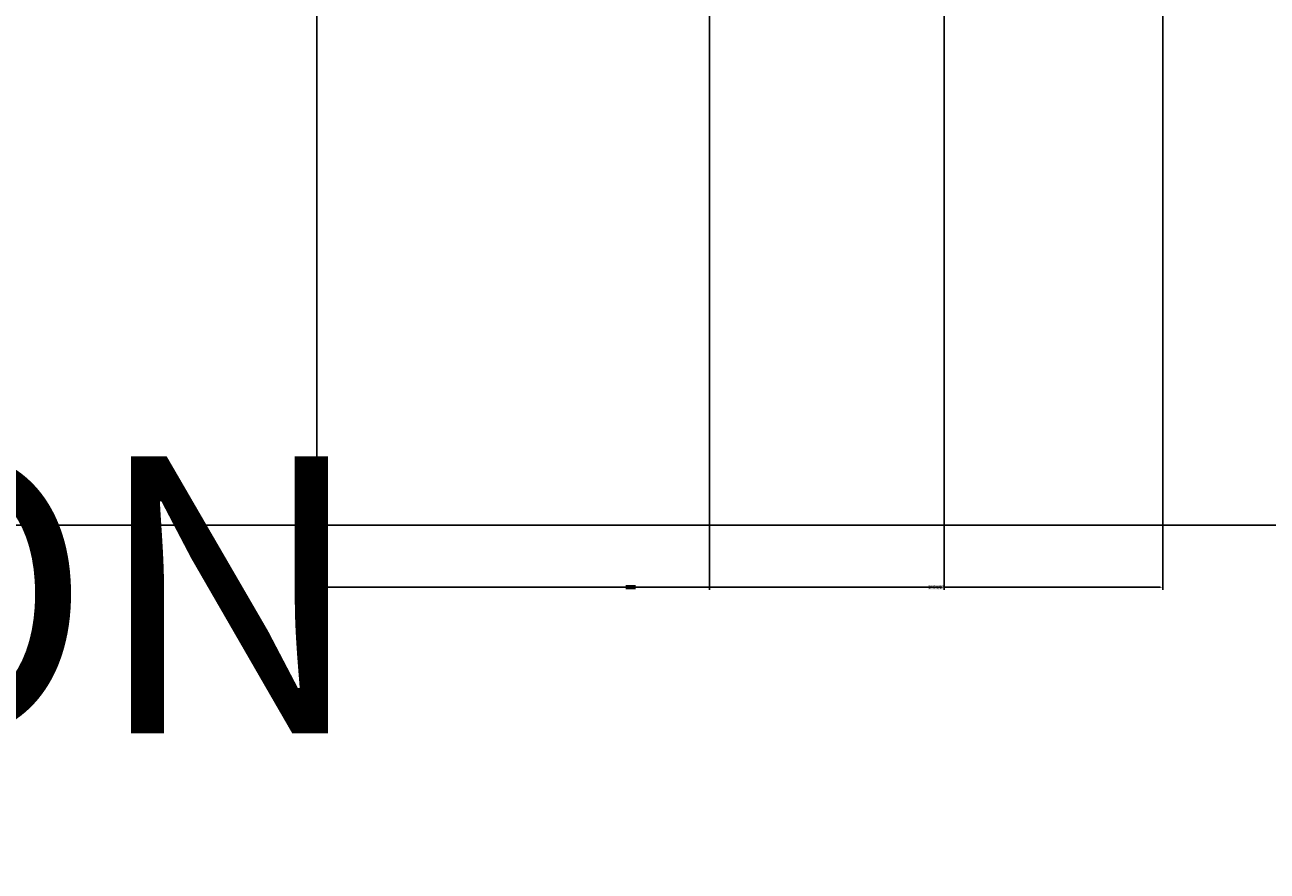
# Model space of a CAD drawing. Units: inches. Extents: x -301 to 715, y -607 to 364.
# Tile 45 of 141: x -17 to 64, y -315 to -260. Entities that reach past the tile are written whole.
import ezdxf

# ---------------------------------------------------------------- set-up
doc = ezdxf.new("R2010")
doc.units = ezdxf.units.IN
doc.header["$MEASUREMENT"] = 0
doc.layers.add('A-ANNO-DIMS', color=2, linetype='Continuous', lineweight=18)
doc.layers.add('A-ANNO-TITL', color=1, linetype='Continuous', lineweight=35)
doc.styles.get("Standard").update_dxf_attribs({"font": 'arial.ttf'})
doc.dimstyles.get("Standard").update_dxf_attribs({"dimtxt": 0.18, "dimasz": 0.18, "dimexe": 0.18, "dimexo": 0.0625, "dimgap": 0.09, "dimtad": 0, "dimtih": 1, "dimtoh": 1, "dimdec": 1, "dimzin": 0, "dimdsep": 46, "dimlunit": 4, "dimtxsty": 'Standard', "dimcen": 0.09, "dimclrd": 3, "dimclre": 4, "dimclrt": 6, "dimadec": 0, "dimazin": 0, "dimtfac": 1, "dimtdec": 1, "dimtofl": 0, "dimtmove": 0, "dimatfit": 3, "dimfxl": 1, "dimtfill": 2, "dimtfillclr": 51, "dimtolj": 1, "dimtzin": 0, "dimarcsym": 0})

# ---------------------------------------------------------------- blocks, each defined once
blk = doc.blocks.new('*D148')
at = {"layer": 'A-ANNO-DIMS', "color": 4, "lineweight": -2, "transparency": 16777216}
for p, q in [((2.397, -223.88), (2.397, -296.865)), ((43.147, -223.88), (43.147, -296.865))]:
    blk.add_line(p, q, dxfattribs=at)
at = {"layer": 'A-ANNO-DIMS', "color": 3, "lineweight": -2, "transparency": 16777216}
for p, q in [((2.577, -296.685), (22.443, -296.685)), ((42.967, -296.685), (23.101, -296.685))]:
    blk.add_line(p, q, dxfattribs=at)
at = {"layer": 'A-ANNO-DIMS', "color": 3, "transparency": 16777216}
for points in [[(2.577, -296.655), (2.577, -296.715), (2.397, -296.685)], [(42.967, -296.655), (42.967, -296.715), (43.147, -296.685)]]:
    blk.add_solid(points, dxfattribs=at)
at = {"layer": 'Defpoints', "color": 0, "transparency": 16777216}
for p in [(2.397, -223.818), (43.147, -223.818), (43.147, -296.685)]:
    blk.add_point(p, dxfattribs=at)
at = {"layer": 'A-ANNO-DIMS', "color": 6, "transparency": 16777216, "insert": (22.772, -296.685), "char_height": 0.18, "attachment_point": 5, "bg_fill": 1, "box_fill_scale": 1.25, "bg_fill_color": 51, "bg_fill_transparency": 0}
blk.add_mtext('\\A1;3\'-5"', dxfattribs=at)
blk = doc.blocks.new('*D160')
at = {"layer": 'A-ANNO-DIMS', "color": 4, "lineweight": -2, "transparency": 16777216}
for p, q in [((57.352, -76.88), (57.352, -296.865)), ((27.897, -78.943), (27.897, -296.865))]:
    blk.add_line(p, q, dxfattribs=at)
at = {"layer": 'A-ANNO-DIMS', "color": 3, "lineweight": -2, "transparency": 16777216}
for p, q in [((28.077, -296.685), (42.084, -296.685)), ((57.172, -296.685), (43.165, -296.685))]:
    blk.add_line(p, q, dxfattribs=at)
at = {"layer": 'A-ANNO-DIMS', "color": 3, "transparency": 16777216}
for points in [[(28.077, -296.655), (28.077, -296.715), (27.897, -296.685)], [(57.172, -296.655), (57.172, -296.715), (57.352, -296.685)]]:
    blk.add_solid(points, dxfattribs=at)
at = {"layer": 'Defpoints', "color": 0, "transparency": 16777216}
for p in [(57.352, -76.818), (27.897, -78.881), (57.352, -296.685)]:
    blk.add_point(p, dxfattribs=at)
at = {"layer": 'A-ANNO-DIMS', "color": 6, "transparency": 16777216, "insert": (42.624, -296.685), "char_height": 0.18, "attachment_point": 5, "bg_fill": 1, "box_fill_scale": 1.25, "bg_fill_color": 51, "bg_fill_transparency": 0}
blk.add_mtext('\\A1;2\'-5 1/2"', dxfattribs=at)
blk = doc.blocks.new('*D175')
at = {"layer": 'A-ANNO-DIMS', "color": 4, "lineweight": -2, "transparency": 16777216}
for p, q in [((-199.282, -324.415), (-199.282, -292.467)), ((148.218, -324.415), (148.218, -292.467))]:
    blk.add_line(p, q, dxfattribs=at)
at = {"layer": 'A-ANNO-DIMS', "color": 3, "lineweight": -2, "transparency": 16777216}
for p, q in [((-199.102, -292.647), (-26.212, -292.647)), ((148.038, -292.647), (-24.852, -292.647))]:
    blk.add_line(p, q, dxfattribs=at)
at = {"layer": 'A-ANNO-DIMS', "color": 3, "transparency": 16777216}
for points in [[(-199.102, -292.617), (-199.102, -292.677), (-199.282, -292.647)], [(148.038, -292.617), (148.038, -292.677), (148.218, -292.647)]]:
    blk.add_solid(points, dxfattribs=at)
at = {"layer": 'Defpoints', "color": 0, "transparency": 16777216}
for p in [(148.218, -292.647), (-199.282, -324.477), (148.218, -324.477)]:
    blk.add_point(p, dxfattribs=at)
at = {"layer": 'A-ANNO-DIMS', "color": 6, "transparency": 16777216, "insert": (-25.532, -292.647), "char_height": 0.18, "attachment_point": 5, "bg_fill": 1, "box_fill_scale": 1.25, "bg_fill_color": 51, "bg_fill_transparency": 0}
blk.add_mtext('\\A1;28\'-11 1/2"', dxfattribs=at)

msp = doc.modelspace()

# ---------------------------------------------------------------- texts
at = {"layer": 'A-ANNO-TITL'}
msp.add_text('SECTION', height=18, dxfattribs=at).set_placement((-97.05, -306.177))

# ---------------------------------------------------------------- dimensions: what is measured, and where the dimension line sits
at = {"layer": 'A-ANNO-DIMS'}
for base, p1, p2, picture, middle in [((57.352, -296.685), (27.897, -78.881), (57.352, -76.818), '*D160', (42.624, -296.685)), ((43.146712, -296.685468), (2.396712, -223.81767), (43.146712, -223.81767), '*D148', (22.771712, -296.685468)), ((148.218, -292.647), (-199.282, -324.477), (148.218, -324.477), '*D175', (-25.532, -292.647))]:
    dim = msp.add_linear_dim(base=base, p1=p1, p2=p2, dimstyle='Standard', override={"dimdec": 1, "dimlfac": 1, "dimrnd": 0, "dimzin": 1, "dimdsep": 46, "dimlunit": 4, "dimfrac": 2}, dxfattribs=at)
    dim.commit()
    dim.dimension.update_dxf_attribs({"geometry": picture, "text_midpoint": middle})

doc.saveas('drawing.dxf')
